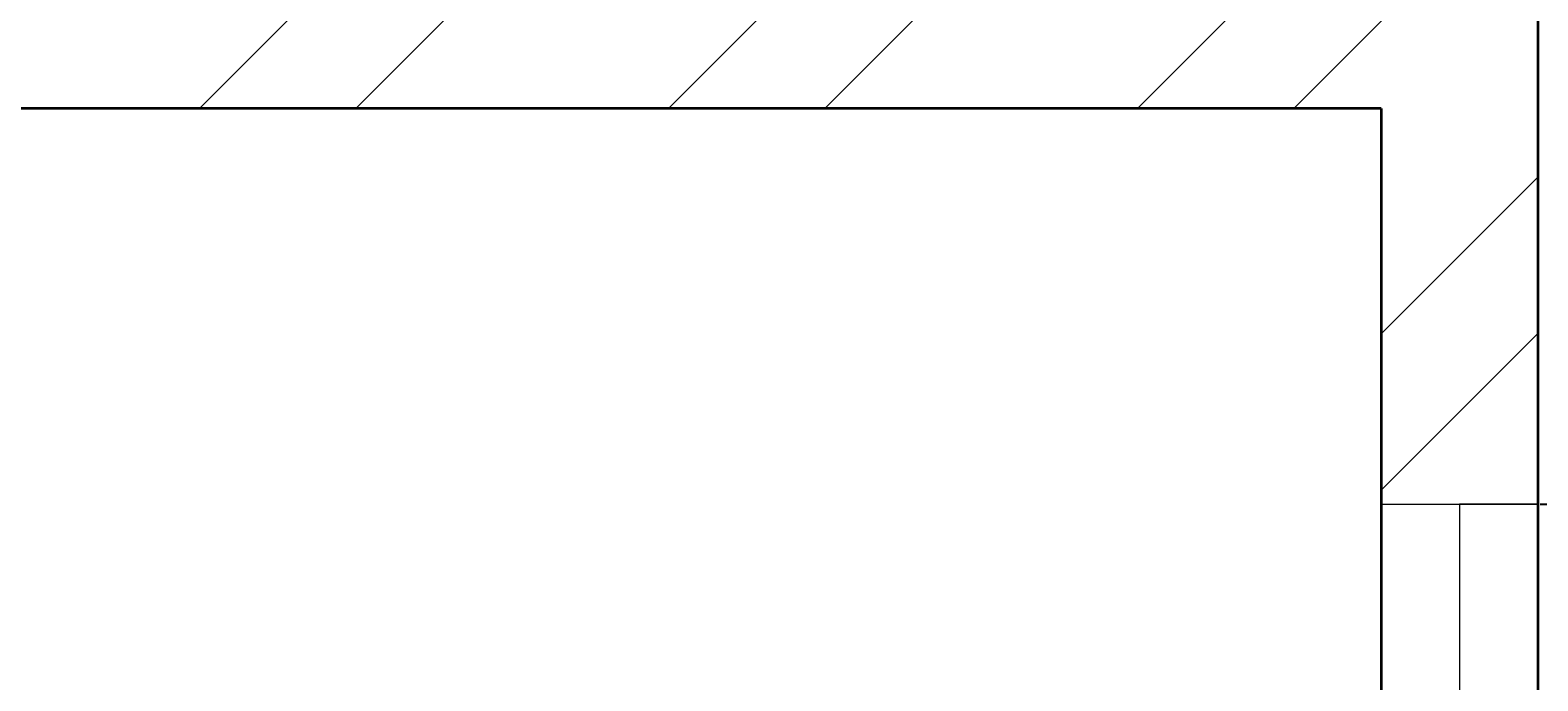
# Model space of a CAD drawing. Units: inches. Extents: x 1962 to 2771, y 1245 to 2660.
# Tile 83 of 114: x 2618 to 2661, y 2161 to 2180. Entities that reach past the tile are written whole.
import ezdxf

# ---------------------------------------------------------------- set-up
doc = ezdxf.new("R2010")
doc.units = ezdxf.units.IN
for name, color, linetype, lineweight in [('A-ANNO-DIMS', 2, 'Continuous', 18), ('A-GLAZ', 4, 'Continuous', 18), ('A-WALL', 7, 'Continuous', 35), ('A-WALL-PATT', 252, 'Continuous', 13)]:
    doc.layers.add(name, color=color, linetype=linetype, lineweight=lineweight)
doc.styles.get("Standard").update_dxf_attribs({"font": 'arial.ttf'})
doc.dimstyles.get("Standard").update_dxf_attribs({"dimtxt": 0.18, "dimasz": 0.18, "dimexe": 0.18, "dimexo": 0.0625, "dimgap": 0.09, "dimtad": 0, "dimtih": 1, "dimtoh": 1, "dimdec": 4, "dimzin": 0, "dimdsep": 46, "dimtxsty": 'Standard', "dimcen": 0.09, "dimadec": 0, "dimazin": 0, "dimtfac": 1, "dimtdec": 4, "dimtofl": 0, "dimtmove": 0, "dimatfit": 3, "dimfxl": 1, "dimtolj": 1, "dimtzin": 0, "dimarcsym": 0})

# ---------------------------------------------------------------- blocks, each defined once
blk = doc.blocks.new('WIN-24IN-B')
for p, q in [((0, 24), (4.5, 24)), ((4.5, 24), (2.25, 24)), ((2.25, 24), (2.25, 0)), ((4.5, 0), (0, 0)), ((2.25, 0), (4.5, 0))]:
    blk.add_line(p, q)
blk = doc.blocks.new('*D20')
at = {"layer": 'A-ANNO-DIMS', "color": 0, "lineweight": -2, "transparency": 16777216}
for p, q in [((2660.87, 2166.485), (2664.587, 2166.485)), ((2664.407, 2166.305), (2664.407, 2154.665)), ((2664.407, 2142.665), (2664.407, 2154.304)), ((2660.87, 2142.485), (2664.587, 2142.485))]:
    blk.add_line(p, q, dxfattribs=at)
at = {"layer": 'A-ANNO-DIMS', "color": 0, "transparency": 16777216}
for points in [[(2664.377, 2166.305), (2664.437, 2166.305), (2664.407, 2166.485)], [(2664.377, 2142.665), (2664.437, 2142.665), (2664.407, 2142.485)]]:
    blk.add_solid(points, dxfattribs=at)
at = {"layer": 'Defpoints', "color": 0, "transparency": 16777216}
for p in [(2660.807, 2166.485), (2664.407, 2166.485), (2660.807, 2142.485)]:
    blk.add_point(p, dxfattribs=at)
at = {"layer": 'A-ANNO-DIMS', "color": 0, "transparency": 16777216, "insert": (2664.407, 2154.485), "char_height": 0.18, "attachment_point": 5}
blk.add_mtext('\\A1;W1B 24 TYP.', dxfattribs=at)
blk = doc.blocks.new('*D40')
at = {"layer": 'A-ANNO-DIMS', "color": 0, "lineweight": -2, "transparency": 16777216}
for p, q in [((2072.02, 2033.906), (2072.02, 2583.474)), ((2072.2, 2583.294), (2366.02, 2583.294)), ((2660.627, 2583.294), (2366.808, 2583.294)), ((2660.807, 2524.406), (2660.807, 2583.474))]:
    blk.add_line(p, q, dxfattribs=at)
at = {"layer": 'A-ANNO-DIMS', "color": 0, "transparency": 16777216}
for points in [[(2072.2, 2583.324), (2072.2, 2583.264), (2072.02, 2583.294)], [(2660.627, 2583.324), (2660.627, 2583.264), (2660.807, 2583.294)]]:
    blk.add_solid(points, dxfattribs=at)
at = {"layer": 'Defpoints', "color": 0, "transparency": 16777216}
for p in [(2660.807, 2583.294), (2660.807, 2524.344), (2072.02, 2033.844)]:
    blk.add_point(p, dxfattribs=at)
at = {"layer": 'A-ANNO-DIMS', "color": 0, "transparency": 16777216, "insert": (2366.414, 2583.294), "char_height": 0.18, "attachment_point": 5}
blk.add_mtext('\\A1;588.8', dxfattribs=at)

msp = doc.modelspace()

# ---------------------------------------------------------------- hatches: boundary and pattern name
at = {"layer": 'A-WALL-PATT'}
h = msp.add_hatch(dxfattribs=at)
h.set_pattern_fill('ANSI32', color=256)
h.paths.add_polyline_path([(2090.8074, 2467.3437), (2141.6481, 2467.3437), (2141.6481, 2469.5937), (2141.6481, 2471.8437), (2086.3074, 2471.8437), (2086.3074, 2422.5333), (2090.8074, 2422.5333)])
h.paths.add_polyline_path([(2282.7664, 2471.8437), (2204.8982, 2471.8437), (2204.8982, 2467.3437), (2234.8074, 2467.3437), (2234.8074, 2311.3437), (2228.7492, 2311.3437), (2228.7492, 2306.8437), (2234.8074, 2306.8437), (2331.9227, 2306.8437), (2331.9227, 2309.0937), (2331.9227, 2311.3437), (2239.3074, 2311.3437), (2239.3074, 2467.3437), (2282.7664, 2467.3437), (2282.7664, 2469.5937)])
h.paths.add_polyline_path([(2471.4531, 2519.8437), (2552.011, 2519.8437), (2564.3996, 2519.8437), (2564.3996, 2511.1389), (2568.8996, 2511.1389), (2568.8996, 2524.3437), (2466.9531, 2524.3437), (2466.9531, 2471.8437), (2450.0749, 2471.8437), (2446.4672, 2471.8437), (2446.4672, 2467.3437), (2450.0749, 2467.3437), (2475.9988, 2467.3437), (2475.9988, 2469.5937), (2475.9988, 2471.8437), (2471.4531, 2471.8437)])
h.paths.add_polyline_path([(2575.2231, 2469.5937), (2575.2231, 2471.8437), (2568.8996, 2471.8437), (2568.8996, 2487.1389), (2564.3996, 2487.1389), (2564.3996, 2471.8437), (2556.511, 2471.8437), (2499.2904, 2471.8437), (2499.2904, 2467.3437), (2507.8074, 2467.3437), (2507.8074, 2311.3437), (2414.863, 2311.3437), (2414.863, 2306.8437), (2512.3074, 2306.8437), (2517.0114, 2306.8437), (2517.0114, 2309.0937), (2517.0114, 2311.3437), (2512.3074, 2311.3437), (2512.3074, 2467.3437), (2575.2231, 2467.3437)])
h.paths.add_polyline_path([(2660.8074, 2471.8437), (2600.9602, 2471.8437), (2600.9602, 2467.3437), (2656.3074, 2467.3437), (2656.3074, 2432.5704), (2660.8074, 2432.5704)])
h.paths.add_polyline_path([(2660.8074, 2372.5704), (2656.3074, 2372.5704), (2656.3074, 2311.3437), (2600.276, 2311.3437), (2600.276, 2309.0937), (2600.276, 2306.8437), (2656.3074, 2306.8437), (2656.3074, 2296.2593), (2660.8074, 2296.2593)])
h.paths.add_polyline_path([(2572.3074, 2306.8437), (2577.1385, 2306.8437), (2577.1385, 2311.3437), (2551.082, 2311.3437), (2551.082, 2306.8437), (2567.8074, 2306.8437), (2567.8074, 2258.8437), (2540.0574, 2258.8437), (2540.0574, 2256.5937), (2540.0574, 2254.3437), (2567.8074, 2254.3437), (2656.3074, 2254.3437), (2656.3074, 2236.9085), (2660.8074, 2236.9085), (2660.8074, 2272.2593), (2656.3074, 2272.2593), (2656.3074, 2258.8437), (2572.3074, 2258.8437)])
h.paths.add_polyline_path([(2512.3074, 2254.3437), (2518.8716, 2254.3437), (2518.8716, 2256.5937), (2518.8716, 2258.8437), (2507.8074, 2258.8437), (2507.8074, 2177.8437), (2567.8074, 2177.8437), (2567.8074, 2172.9628), (2572.3074, 2172.9628), (2572.3074, 2177.8437), (2656.3074, 2177.8437), (2656.3074, 2166.4846), (2660.8074, 2166.4846), (2660.8074, 2200.9085), (2656.3074, 2200.9085), (2656.3074, 2182.3437), (2512.3074, 2182.3437)])
h.paths.add_polyline_path([(2656.3074, 2129.8437), (2572.3074, 2129.8437), (2572.3074, 2150.3044), (2570.0574, 2150.3044), (2567.8074, 2150.3044), (2567.8074, 2129.8437), (2507.8074, 2129.8437), (2507.8074, 2116.3027), (2510.0574, 2116.3027), (2512.3074, 2116.3027), (2512.3074, 2125.3437), (2567.8074, 2125.3437), (2572.3074, 2125.3437), (2656.3074, 2125.3437)])
h.paths.add_polyline_path([(2090.8074, 2362.5333), (2086.3074, 2362.5333), (2086.3074, 2298.6242), (2090.8074, 2298.6242), (2090.8074, 2306.8437), (2174.8074, 2306.8437), (2174.8074, 2286.4178), (2179.3074, 2286.4178), (2179.3074, 2306.8437), (2192.8641, 2306.8437), (2192.8641, 2309.0937), (2192.8641, 2311.3437), (2090.8074, 2311.3437)])
h.paths.add_polyline_path([(2209.156, 2258.8437), (2179.3074, 2258.8437), (2179.3074, 2263.2236), (2177.0574, 2263.2236), (2174.8074, 2263.2236), (2174.8074, 2258.8437), (2090.8074, 2258.8437), (2090.8074, 2274.6242), (2086.3074, 2274.6242), (2086.3074, 2238.2967), (2088.5574, 2238.2967), (2090.8074, 2238.2967), (2090.8074, 2254.3437), (2209.156, 2254.3437)])
h.paths.add_polyline_path([(2090.8074, 2177.8437), (2234.8074, 2177.8437), (2234.8074, 2173.1428), (2239.3074, 2173.1428), (2239.3074, 2258.8437), (2230.8442, 2258.8437), (2230.8442, 2256.5937), (2230.8442, 2254.3437), (2234.8074, 2254.3437), (2234.8074, 2182.3437), (2090.8074, 2182.3437), (2090.8074, 2202.2967), (2086.3074, 2202.2967), (2086.3074, 2140.0389), (2090.8074, 2140.0389)])
h.paths.add_polyline_path([(2090.8074, 2080.0389), (2086.3074, 2080.0389), (2086.3074, 2033.8437), (2090.8074, 2033.8437)], flags=17)
h.paths.add_polyline_path([(2244.9405, 2033.8437), (2239.3074, 2033.8437), (2239.3074, 2142.0665), (2237.2592, 2142.0665), (2234.8074, 2142.0665), (2234.8074, 2033.8437), (2090.8074, 2033.8437), (2076.5204, 2033.8437), (2072.0204, 2033.8437), (2072.0204, 2000.4493), (2076.5204, 2000.4493), (2076.5204, 2029.3437), (2090.8074, 2029.3437), (2244.9405, 2029.3437), (2244.9405, 2031.5937)])
h.paths.add_polyline_path([(2234.8074, 1933.3437), (2076.5204, 1933.3437), (2076.5204, 1952.4493), (2074.2704, 1952.4493), (2072.0204, 1952.4493), (2072.0204, 1933.3437), (2072.0204, 1928.8437), (2234.8074, 1928.8437)])
h.paths.add_polyline_path([(2090.8074, 1928.8437), (2086.3074, 1928.8437), (2086.3074, 1906.5013), (2090.8074, 1906.5013)])
h.paths.add_polyline_path([(2090.8074, 1846.5013), (2086.3074, 1846.5013), (2086.3074, 1769.9917), (2088.5574, 1769.9917), (2090.8074, 1769.9917), (2090.8074, 1780.3437), (2234.8074, 1780.3437), (2234.8074, 1708.3437), (2230.3764, 1708.3437), (2230.3764, 1703.8437), (2239.3074, 1703.8437), (2239.3074, 1792.6669), (2237.0574, 1792.6669), (2234.8074, 1792.6669), (2234.8074, 1784.8437), (2090.8074, 1784.8437)])
h.paths.add_polyline_path([(2239.3074, 1928.8437), (2244.9405, 1928.8437), (2244.9405, 1931.0937), (2244.9405, 1933.3437), (2234.8074, 1933.3437), (2234.8074, 1928.8437), (2234.8074, 1825.5949), (2239.3074, 1825.5949)])
h.paths.add_polyline_path([(2148.0425, 1649.0937), (2148.0425, 1651.3437), (2090.8074, 1651.3437), (2090.8074, 1646.8437), (2148.0425, 1646.8437)], flags=0)
h.paths.add_polyline_path([(2207.5601, 1708.3437), (2090.8074, 1708.3437), (2090.8074, 1703.8437), (2174.8074, 1703.8437), (2174.8074, 1651.3437), (2170.4457, 1651.3437), (2170.4457, 1646.8437), (2195.9924, 1646.8437), (2195.9924, 1649.0937), (2195.9924, 1651.3437), (2179.3074, 1651.3437), (2179.3074, 1703.8437), (2207.5601, 1703.8437), (2207.5601, 1706.0937)])
h.paths.add_polyline_path([(2090.8074, 1733.9917), (2086.3074, 1733.9917), (2086.3074, 1696.1032), (2088.5574, 1696.1032), (2090.8074, 1696.1032)])
h.paths.add_polyline_path([(2090.8074, 1672.1032), (2086.3074, 1672.1032), (2086.3074, 1600.3335), (2090.8074, 1600.3335)])
h.paths.add_polyline_path([(2090.8074, 1540.3335), (2086.3074, 1540.3335), (2086.3074, 1486.3437), (2139.6766, 1486.3437), (2139.6766, 1490.8437), (2090.8074, 1490.8437)])
h.paths.add_polyline_path([(2302.3876, 1490.8437), (2239.3074, 1490.8437), (2239.3074, 1646.8437), (2335.9994, 1646.8437), (2335.9994, 1651.3437), (2229.884, 1651.3437), (2229.884, 1646.8437), (2234.8074, 1646.8437), (2234.8074, 1490.8437), (2202.7103, 1490.8437), (2202.7103, 1488.5937), (2202.7103, 1486.3437), (2275.0699, 1486.3437), (2275.0699, 1475.772), (2279.5699, 1475.772), (2279.5699, 1486.3437), (2302.3876, 1486.3437)])
h.paths.add_polyline_path([(2279.5699, 1451.772), (2275.0699, 1451.772), (2275.0699, 1438.3437), (2174.8074, 1438.3437), (2174.8074, 1486.3437), (2179.7922, 1486.3437), (2179.7922, 1490.8437), (2163.3585, 1490.8437), (2163.3585, 1488.5937), (2163.3585, 1486.3437), (2170.3074, 1486.3437), (2170.3074, 1433.8437), (2279.5699, 1433.8437)])
h.paths.add_polyline_path([(2427.2363, 1490.8437), (2375.8074, 1490.8437), (2375.8074, 1646.8437), (2381.6401, 1646.8437), (2381.6401, 1651.3437), (2365.887, 1651.3437), (2365.887, 1649.0937), (2365.887, 1646.8437), (2371.3074, 1646.8437), (2371.3074, 1490.8437), (2327.5627, 1490.8437), (2327.5627, 1488.5937), (2327.5627, 1486.3437), (2371.3074, 1486.3437), (2371.3074, 1433.8437), (2375.8074, 1433.8437), (2375.8074, 1486.3437), (2427.2363, 1486.3437)])
h.paths.add_polyline_path([(2512.3074, 1646.8437), (2519.4351, 1646.8437), (2519.4351, 1649.0937), (2519.4351, 1651.3437), (2507.8074, 1651.3437), (2416.0063, 1651.3437), (2416.0063, 1649.0937), (2416.0063, 1646.8437), (2507.8074, 1646.8437), (2507.8074, 1490.8437), (2497.0532, 1490.8437), (2497.0532, 1488.5937), (2497.0532, 1486.3437), (2574.9344, 1486.3437), (2574.9344, 1476.0181), (2579.4344, 1476.0181), (2579.4344, 1486.3437), (2584.4872, 1486.3437), (2584.3074, 1490.8437), (2512.3074, 1490.8437)])
h.paths.add_polyline_path([(2470.5091, 1486.3437), (2473.9767, 1486.3437), (2473.9767, 1490.8437), (2449.6605, 1490.8437), (2449.6605, 1488.5937), (2449.6605, 1486.3437), (2466.0091, 1486.3437), (2466.0091, 1433.8437), (2470.5091, 1433.8437), (2579.4344, 1433.8437), (2579.4344, 1452.0181), (2574.9344, 1452.0181), (2574.9344, 1438.3437), (2554.5091, 1438.3437), (2470.5091, 1438.3437)])
h.paths.add_polyline_path([(2656.3074, 1490.8437), (2611.86, 1490.8437), (2611.86, 1486.3437), (2656.3074, 1486.3437)])
h.paths.add_polyline_path([(2660.8074, 1532.7007), (2658.5574, 1532.7007), (2656.3074, 1532.7007), (2656.3074, 1486.3437), (2660.8074, 1486.3437)])
h.paths.add_polyline_path([(2660.8074, 1664.9663), (2656.3074, 1664.9663), (2656.3074, 1651.3437), (2602.2313, 1651.3437), (2602.2313, 1646.8437), (2656.3074, 1646.8437), (2656.3074, 1592.7007), (2660.8074, 1592.7007)])
h.paths.add_polyline_path([(2660.8074, 1724.5221), (2656.3074, 1724.5221), (2656.3074, 1703.8437), (2542.4725, 1703.8437), (2542.4725, 1699.3437), (2567.8074, 1699.3437), (2567.8074, 1651.3437), (2552.7766, 1651.3437), (2552.7766, 1649.0937), (2552.7766, 1646.8437), (2577.2878, 1646.8437), (2577.2878, 1649.0937), (2577.2878, 1651.3437), (2572.3074, 1651.3437), (2572.3074, 1699.3437), (2656.3074, 1699.3437), (2656.3074, 1688.9663), (2660.8074, 1688.9663)])
h.paths.add_polyline_path([(2660.8074, 1880.6524), (2656.3074, 1880.6524), (2656.3074, 1832.8437), (2512.3074, 1832.8437), (2512.3074, 1837.8959), (2507.8074, 1837.8959), (2507.8074, 1828.3437), (2567.8074, 1828.3437), (2567.8074, 1804.3437), (2572.3074, 1804.3437), (2572.3074, 1828.3437), (2656.3074, 1828.3437), (2656.3074, 1818.6778), (2660.8074, 1818.6778)])
h.paths.add_polyline_path([(2660.8074, 1794.6778), (2656.3074, 1794.6778), (2656.3074, 1780.3437), (2572.3074, 1780.3437), (2572.3074, 1783.0303), (2570.0574, 1783.0303), (2567.8074, 1783.0303), (2567.8074, 1780.3437), (2507.8074, 1780.3437), (2507.8074, 1699.3437), (2517.8858, 1699.3437), (2517.8858, 1701.5937), (2517.8858, 1703.8437), (2512.3074, 1703.8437), (2512.3074, 1775.8437), (2656.3074, 1775.8437), (2656.3074, 1760.5221), (2660.8074, 1760.5221)])
h.paths.add_polyline_path([(2660.8074, 1981.3437), (2660.8074, 2020.2808), (2658.5574, 2020.2808), (2656.3074, 2020.2808), (2656.3074, 1981.3437), (2512.3074, 1981.3437), (2512.3074, 2086.6996), (2507.8074, 2086.6996), (2507.8074, 1981.3437), (2375.8074, 1981.3437), (2375.8074, 1986.8505), (2373.5574, 1986.8505), (2371.3074, 1986.8505), (2371.3074, 1973.2607), (2375.8074, 1973.2607), (2375.8074, 1976.8437), (2507.8074, 1976.8437), (2507.8074, 1865.4281), (2510.0574, 1865.4281), (2512.3074, 1865.4281), (2512.3074, 1976.8437), (2660.8074, 1976.8437)])
h.paths.add_polyline_path([(2375.8074, 1940.297), (2373.5574, 1940.297), (2371.3074, 1940.297), (2371.3074, 1933.3437), (2278.4434, 1933.3437), (2278.4434, 1928.8437), (2371.3074, 1928.8437), (2371.3074, 1651.3437), (2375.8074, 1651.3437)])
h.paths.add_polyline_path([(2660.8074, 1976.8437), (2656.3074, 1976.8437), (2656.3074, 1940.6524), (2660.8074, 1940.6524)], flags=17)
h.paths.add_polyline_path([(2660.8074, 2142.4846), (2656.3074, 2142.4846), (2656.3074, 2080.2808), (2660.8074, 2080.2808)])
h.paths.add_polyline_path([(2381.4189, 2311.3437), (2375.8074, 2311.3437), (2375.8074, 2467.3437), (2424.7242, 2467.3437), (2424.7242, 2469.5937), (2424.7242, 2471.8437), (2375.8074, 2471.8437), (2375.8074, 2524.3437), (2371.3074, 2524.3437), (2371.3074, 2471.8437), (2307.2097, 2471.8437), (2307.2097, 2467.3437), (2371.3074, 2467.3437), (2371.3074, 2311.3437), (2366.8901, 2311.3437), (2366.8901, 2306.8437), (2371.3074, 2306.8437), (2371.3074, 2033.8437), (2279.6589, 2033.8437), (2279.6589, 2029.3437), (2371.3074, 2029.3437), (2371.3074, 2014.2598), (2375.8074, 2014.2598), (2375.8074, 2306.8437), (2381.4189, 2306.8437)])
h.paths.add_polyline_path([(2263.3074, 2524.3437), (2170.3074, 2524.3437), (2170.3074, 2519.8437), (2170.3074, 2471.8437), (2165.0312, 2471.8437), (2165.0312, 2467.3437), (2179.6721, 2467.3437), (2179.6721, 2469.5161), (2179.6721, 2471.8437), (2174.8074, 2471.8437), (2174.8074, 2519.8437), (2258.8074, 2519.8437), (2258.8074, 2511.6436), (2263.3074, 2511.6436)])
h.paths.add_polyline_path([(2245.0232, 1361.4123), (2492.9468, 1361.4123), (2492.9468, 1398.505), (2245.0232, 1398.505)], flags=9)
h.paths.add_polyline_path([(2388.1434, 2086.6936), (2425.0704, 2086.6936), (2425.0704, 2105.3509), (2388.1434, 2105.3509)], flags=9)
h.paths.add_polyline_path([(2404.922, 2242.6744), (2445.7337, 2242.6744), (2445.7337, 2261.3318), (2404.922, 2261.3318)], flags=9)
h.paths.add_polyline_path([(2269.4107, 2156.7935), (2306.3378, 2156.7935), (2306.3378, 2175.4508), (2269.4107, 2175.4508)], flags=9)
h.paths.add_polyline_path([(2269.3277, 2233.4343), (2306.2547, 2233.4343), (2306.2547, 2252.0917), (2269.3277, 2252.0917)], flags=9)
h.paths.add_polyline_path([(2431.6052, 2320.6922), (2470.4456, 2320.6922), (2470.4456, 2339.3495), (2431.6052, 2339.3495)], flags=25)
h.paths.add_polyline_path([(2249.6902, 2315.7608), (2288.5306, 2315.7608), (2288.5306, 2334.4182), (2249.6902, 2334.4182)], flags=25)
h.paths.add_polyline_path([(2096.9301, 2314.3181), (2135.7704, 2314.3181), (2135.7704, 2332.9755), (2096.9301, 2332.9755)], flags=25)
h.paths.add_polyline_path([(2134.3475, 2285.7089), (2161.4655, 2285.7089), (2161.4655, 2304.3662), (2134.3475, 2304.3662)], flags=9)
h.paths.add_polyline_path([(2126.5155, 2209.4076), (2159.9227, 2209.4076), (2159.9227, 2228.065), (2126.5155, 2228.065)], flags=25)
h.paths.add_polyline_path([(2110.5753, 2141.5299), (2149.4157, 2141.5299), (2149.4157, 2160.1872), (2110.5753, 2160.1872)], flags=25)
h.paths.add_polyline_path([(2249.8618, 1968.3317), (2286.3966, 1968.3317), (2286.3966, 1986.989), (2249.8618, 1986.989)], flags=9)
h.paths.add_polyline_path([(2395.9507, 1777.0051), (2436.7624, 1777.0051), (2436.7624, 1795.6625), (2395.9507, 1795.6625)], flags=9)
h.paths.add_polyline_path([(2398.5259, 1888.5651), (2435.0062, 1888.5651), (2435.0062, 1907.2224), (2398.5259, 1907.2224)], flags=25)
h.paths.add_polyline_path([(2259.3506, 1728.3559), (2296.2776, 1728.3559), (2296.2776, 1747.0132), (2259.3506, 1747.0132)], flags=9)
h.paths.add_polyline_path([(2271.3698, 1845.268), (2308.2968, 1845.268), (2308.2968, 1863.9253), (2271.3698, 1863.9253)], flags=9)
h.paths.add_polyline_path([(2120.9355, 1786.3027), (2159.7759, 1786.3027), (2159.7759, 1804.9601), (2120.9355, 1804.9601)], flags=25)
h.paths.add_polyline_path([(2121.3164, 1732.1043), (2154.7236, 1732.1043), (2154.7236, 1750.7616), (2121.3164, 1750.7616)], flags=25)
h.paths.add_polyline_path([(2118.3706, 1678.8997), (2147.5282, 1678.8997), (2147.5282, 1697.557), (2118.3706, 1697.557)], flags=25)
h.paths.add_polyline_path([(2385.9227, 1493.557), (2424.763, 1493.557), (2424.763, 1512.2143), (2385.9227, 1512.2143)], flags=25)
h.paths.add_polyline_path([(2248.7058, 1500.0256), (2287.5462, 1500.0256), (2287.5462, 1518.6829), (2248.7058, 1518.6829)], flags=25)
h.paths.add_polyline_path([(2104.1669, 1617.3771), (2143.0073, 1617.3771), (2143.0073, 1636.0344), (2104.1669, 1636.0344)], flags=9)
h.paths.add_polyline_path([(2096.0714, 1447.8824), (2137.3845, 1447.8824), (2137.3845, 1458.1859), (2096.0714, 1458.1859)], flags=9)
h.paths.add_polyline_path([(2180.6114, 1440.325), (2209.7689, 1440.325), (2209.7689, 1458.9823), (2180.6114, 1458.9823)], flags=25)
h.paths.add_polyline_path([(2316.1698, 1447.9637), (2357.4829, 1447.9637), (2357.4829, 1458.2673), (2316.1698, 1458.2673)], flags=9)
h.paths.add_polyline_path([(2397.6187, 1447.9637), (2438.9318, 1447.9637), (2438.9318, 1458.2673), (2397.6187, 1458.2673)], flags=9)
h.paths.add_polyline_path([(2473.0778, 1439.5953), (2502.2354, 1439.5953), (2502.2354, 1458.2527), (2473.0778, 1458.2527)], flags=25)
h.paths.add_polyline_path([(2589.7027, 1447.8819), (2631.0158, 1447.8819), (2631.0158, 1458.1855), (2589.7027, 1458.1855)], flags=9)
h.paths.add_polyline_path([(2522.4009, 1497.5285), (2561.2413, 1497.5285), (2561.2413, 1516.1859), (2522.4009, 1516.1859)], flags=25)
h.paths.add_polyline_path([(2579.6565, 1671.3482), (2608.8141, 1671.3482), (2608.8141, 1690.0056), (2579.6565, 1690.0056)], flags=25)
h.paths.add_polyline_path([(2544.7038, 1725.5064), (2578.1111, 1725.5064), (2578.1111, 1744.1637), (2544.7038, 1744.1637)], flags=25)
h.paths.add_polyline_path([(2578.1191, 1807.472), (2607.2766, 1807.472), (2607.2766, 1826.1293), (2578.1191, 1826.1293)], flags=25)
h.paths.add_polyline_path([(2595.0614, 1835.1839), (2633.9018, 1835.1839), (2633.9018, 1853.8413), (2595.0614, 1853.8413)], flags=25)
h.paths.add_polyline_path([(2567.0097, 2097.7035), (2605.8501, 2097.7035), (2605.8501, 2116.3609), (2567.0097, 2116.3609)], flags=9)
h.paths.add_polyline_path([(2586.644, 2134.6454), (2615.8015, 2134.6454), (2615.8015, 2153.3027), (2586.644, 2153.3027)], flags=9)
h.paths.add_polyline_path([(2544.6185, 2212.6783), (2578.0258, 2212.6783), (2578.0258, 2231.3356), (2544.6185, 2231.3356)], flags=25)
h.paths.add_polyline_path([(2577.0273, 2256.9023), (2606.1849, 2256.9023), (2606.1849, 2275.5597), (2577.0273, 2275.5597)], flags=24)
h.paths.add_polyline_path([(2605.2683, 2315.2821), (2644.1087, 2315.2821), (2644.1087, 2333.9395), (2605.2683, 2333.9395)], flags=25)
h.paths.add_polyline_path([(2583.1244, 2496.1815), (2624.4375, 2496.1815), (2624.4375, 2506.4851), (2583.1244, 2506.4851)], flags=9)
h.paths.add_polyline_path([(2474.761, 2497.0823), (2503.9185, 2497.0823), (2503.9185, 2515.7397), (2474.761, 2515.7397)], flags=25)
h.paths.add_polyline_path([(2387.5787, 2494.2563), (2428.902, 2494.2563), (2428.902, 2504.5598), (2387.5787, 2504.5598)], flags=9)
h.paths.add_polyline_path([(2300.1657, 2500.1564), (2341.4788, 2500.1564), (2341.4788, 2510.46), (2300.1657, 2510.46)], flags=25)
h.paths.add_polyline_path([(2176.8589, 2497.5843), (2206.0165, 2497.5843), (2206.0165, 2516.2416), (2176.8589, 2516.2416)], flags=25)
h.paths.add_polyline_path([(2097.4668, 2494.9762), (2138.7799, 2494.9762), (2138.7799, 2505.2798), (2097.4668, 2505.2798)], flags=9)

# ---------------------------------------------------------------- linework, layer by layer
at = {"layer": 'A-WALL'}
for p, q in [((2660.8074, 2471.8437), (2660.8074, 1976.8437)), ((2656.3074, 2177.8437), (2572.3074, 2177.8437)), ((2656.3074, 2177.8437), (2572.3074, 2177.8437)), ((2656.3074, 2177.8437), (2656.3074, 1981.3437))]:
    msp.add_line(p, q, dxfattribs=at)

# ---------------------------------------------------------------- block references
at = {"layer": 'A-GLAZ'}
msp.add_blockref('WIN-24IN-B', (2656.3074, 2142.4846), dxfattribs=at)

# ---------------------------------------------------------------- dimensions: what is measured, and where the dimension line sits
at = {"layer": 'A-ANNO-DIMS'}
dim = msp.add_linear_dim(base=(2660.8074, 2583.2937), p1=(2072.0204, 2033.8437), p2=(2660.8074, 2524.3437), dimstyle='Standard', override={"dimdec": 1, "dimlfac": 1, "dimrnd": 0, "dimzin": 0, "dimdsep": 46, "dimlunit": 2}, dxfattribs=at)
dim.commit()
dim.dimension.update_dxf_attribs({"geometry": '*D40', "text_midpoint": (2366.4139, 2583.2937)})
dim = msp.add_linear_dim(base=(2664.4074, 2166.4846), p1=(2660.8074, 2142.4846), p2=(2660.8074, 2166.4846), angle=90, text='W1B <> TYP.', dimstyle='Standard', override={"dimdec": 0, "dimlfac": 1, "dimrnd": 0, "dimzin": 0, "dimdsep": 46, "dimlunit": 2}, dxfattribs=at)
dim.commit()
dim.dimension.update_dxf_attribs({"geometry": '*D20', "text_midpoint": (2664.4074, 2154.4846)})

doc.saveas('drawing.dxf')
